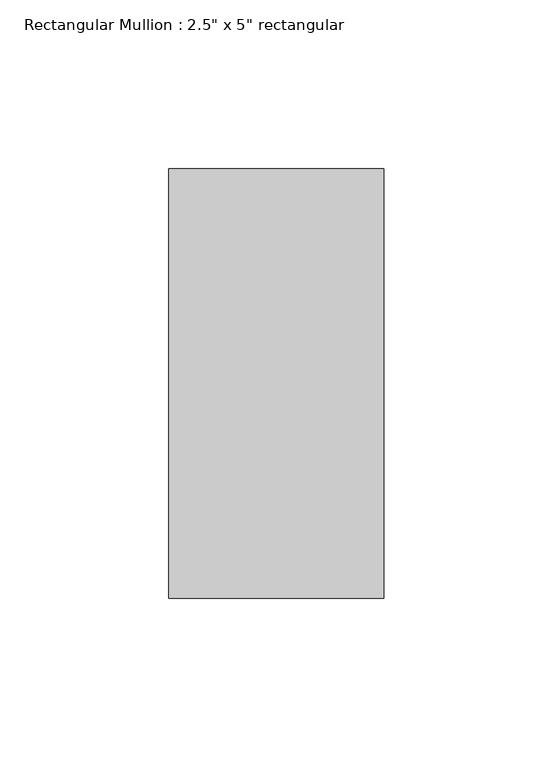
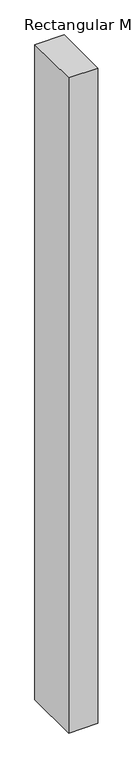
"""IFC4 building model written with IfcOpenShell, lengths in millimetres: member geometry."""

from ifc_helpers import new_model, si_unit, frame, origin, place, context, project, spatial, polyline, outline, extrude, source, transform, mapped, element, save


def member_1b4b4554(model_context):
    return source(origin(), model_context, "Body", "SweptSolid", [
        extrude(outline(polyline([(31.75, 63.5), (31.75, -63.5), (-31.75, -63.5), (-31.75, 63.5), (31.75, 63.5)])), frame((0.0, 0.0, -1509.6020555), z_axis=(0.0, 0.0, 1.0), x_axis=(1.0, 0.0, 0.0)), (0.0, 0.0, 1.0), 1509.6020555),
    ])


if __name__ == "__main__":
    model = new_model("IFC4")
    model_context = context("Model", 3, world=origin())
    ifc_project = project(units=[si_unit("LENGTHUNIT", "METRE", prefix="MILLI")], contexts=[model_context])
    site = spatial("IfcSite", under=ifc_project)
    building = spatial("IfcBuilding", under=site)
    placement = place(None, origin())
    member_shape = member_1b4b4554(model_context)
    element("IfcMember", 1, ObjectType="Rectangular Mullion : 2.5\" x 5\" rectangular", at=placement, inside=building, context=model_context, shape_type="MappedRepresentation", body=[
        mapped(member_shape, transform((0.0, 0.0, 0.0), x_axis=(1.0, 0.0, 0.0), y_axis=(0.0, 1.0, 0.0), z_axis=(0.0, 0.0, 1.0))),
    ])
    save(model, "model.ifc")

# Revit data of these elements
# Type "Rectangular Mullion : 2.5\" x 5\" rectangular"
#   built-in parameter 1007304 = 0.416667 (stored number, unit not read)
#   built-in parameter 1007301 = 0.104167 (stored number, unit not read)
#   built-in parameter 1007300 = 0.104167 (stored number, unit not read)
# Element 1 (IfcMember, "Rectangular Mullion : 2.5\" x 5\" rectangular")
#   Materials on its faces: "Aluminum"
# Materials
#   "Aluminum": class "Metal", colour RGB 247 247 247, transparency 0, Description = "Aluminum 6061", Cost = 0
